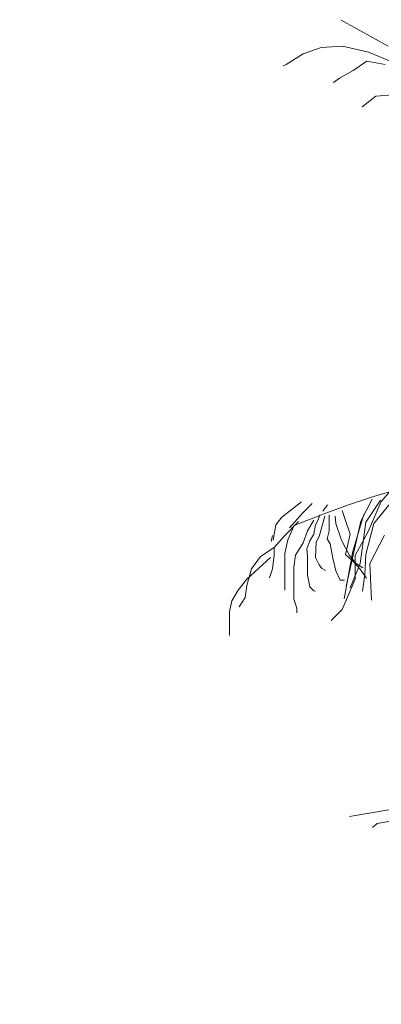
# Model space of a CAD drawing. Units: millimetres. Extents: x 595116 to 630915, y 909473 to 920225.
# Tile 33 of 134: x 629654.1 to 629660.18, y 919163.95 to 919180.52. Entities that reach past the tile are written whole.
import ezdxf

# ---------------------------------------------------------------- set-up
doc = ezdxf.new("R2010")
doc.units = ezdxf.units.MM
doc.layers.add('Dimension', color=3, linetype='Continuous', lineweight=18)
doc.layers.add('L-PLNT', color=85, linetype='Continuous', lineweight=13)
doc.styles.get("Standard").update_dxf_attribs({"font": 'arial.ttf'})
doc.dimstyles.new('ISO-25', dxfattribs={"dimtxt": 9, "dimasz": 6, "dimexe": 1.25, "dimexo": 0.625, "dimtad": 1, "dimlunit": 4, "dimtxsty": 'Standard', "dimcen": 2.5, "dimadec": 0, "dimazin": 0, "dimtfac": 1, "dimtmove": 0, "dimatfit": 3, "dimfxl": 1, "dimarcsym": 0})

# ---------------------------------------------------------------- blocks, each defined once
blk = doc.blocks.new('A$C4FB75ABC')
for p, q in [((0.4999, 4.2779), (0.7111, 4.1621)), ((0.4114, 4.1553), (0.3296, 4.1281)), ((0.5068, 4.1621), (0.4114, 4.1553)), ((0.6226, 4.1349), (0.5068, 4.1621)), ((0.3296, 4.1281), (0.2547, 4.0804)), ((0.7861, 4.0668), (0.6226, 4.1349)), ((0.2547, 4.0804), (0.241, 4.0736)), ((0.6158, 4.094), (0.5544, 4.0532)), ((0.6975, 4.0804), (0.6158, 4.094)), ((0.4931, 4.0191), (0.4659, 3.9987)), ((0.5544, 4.0532), (0.4931, 4.0191)), ((0.6566, 3.9374), (0.5953, 3.8897)), ((0.7316, 3.9442), (0.6566, 3.9374)), ((0.7572, 2.2091), (0.6795, 2.1218)), ((0.7422, 2.1723), (0.6405, 2.1416)), ((0.2683, 2.0784), (0.3228, 2.1193)), ((0.6405, 2.1416), (0.5342, 2.1057)), ((0.64, 2.1313), (0.5889, 2.0328)), ((0.6765, 2.1276), (0.6108, 2.0291)), ((0.6795, 2.1218), (0.6213, 1.986)), ((0.7531, 2.1531), (0.6473, 2.0218)), ((0.2342, 2.0512), (0.2683, 2.0784)), ((0.3296, 2.0716), (0.3705, 2.1125)), ((0.4182, 2.0784), (0.4386, 2.1057)), ((0.5342, 2.1057), (0.4195, 2.0639)), ((0.505, 2.0802), (0.5196, 2.0364)), ((0.207, 2.0172), (0.2342, 2.0512)), ((0.3092, 2.0308), (0.2479, 1.9695)), ((0.2683, 2.0035), (0.3296, 2.0716)), ((0.4195, 2.0639), (0.2927, 2.0154)), ((0.3773, 2.0376), (0.3501, 1.9899)), ((0.3966, 2.0361), (0.3855, 2.0168)), ((0.4049, 2.0609), (0.3966, 2.0361)), ((0.427, 2.0554), (0.4021, 1.9643)), ((0.4463, 2.0609), (0.4463, 1.9892)), ((0.4739, 2.0554), (0.4767, 2.0223)), ((0.5196, 2.0364), (0.5415, 1.9744)), ((0.5889, 2.0328), (0.5232, 1.741)), ((0.6018, 2.0636), (0.5533, 1.8986)), ((0.195, 1.9478), (0.207, 2.0172)), ((0.2887, 2.0103), (0.2615, 1.9491)), ((0.3501, 1.9899), (0.3296, 1.9354)), ((0.3855, 2.0168), (0.3773, 1.9754)), ((0.4463, 1.9892), (0.438, 1.9533)), ((0.4767, 2.0223), (0.5015, 1.9478)), ((0.6213, 1.986), (0.563, 1.8792)), ((0.6108, 2.0291), (0.5853, 1.8431)), ((0.6473, 2.0218), (0.6108, 1.8833)), ((0.1865, 1.9422), (0.1934, 1.9695)), ((0.2479, 1.9695), (0.2002, 1.915)), ((0.2615, 1.9491), (0.2479, 1.8878)), ((0.3607, 1.945), (0.3469, 1.9091)), ((0.3773, 1.9754), (0.3607, 1.945)), ((0.4021, 1.9643), (0.3883, 1.9395)), ((0.438, 1.9533), (0.4518, 1.9312)), ((0.5015, 1.9478), (0.5374, 1.8788)), ((0.5415, 1.9744), (0.5196, 1.8833)), ((0.6947, 1.9708), (0.629, 1.8431)), ((0.2002, 1.915), (0.1389, 1.8742)), ((0.2002, 1.915), (0.2002, 1.881)), ((0.3296, 1.9354), (0.2956, 1.881)), ((0.3469, 1.9091), (0.3497, 1.876)), ((0.3883, 1.9395), (0.3855, 1.8705)), ((0.4518, 1.9312), (0.4629, 1.8677)), ((0.5533, 1.8986), (0.5339, 1.7919)), ((0.1844, 1.8695), (0.0777, 1.7725)), ((0.1389, 1.8742), (0.098, 1.8197)), ((0.2002, 1.881), (0.1934, 1.8197)), ((0.2479, 1.8878), (0.2479, 1.8061)), ((0.2956, 1.881), (0.2887, 1.8265)), ((0.3497, 1.876), (0.3497, 1.8512)), ((0.3855, 1.8705), (0.4021, 1.8374)), ((0.4629, 1.8677), (0.4767, 1.8098)), ((0.5196, 1.8833), (0.5524, 1.8541)), ((0.5374, 1.8788), (0.5678, 1.8429)), ((0.5524, 1.8541), (0.5853, 1.8176)), ((0.563, 1.8792), (0.563, 1.7725)), ((0.6108, 1.8833), (0.6072, 1.7957)), ((0.098, 1.8197), (0.0775, 1.7448)), ((0.1934, 1.8197), (0.1797, 1.7788)), ((0.2887, 1.8265), (0.2887, 1.7516)), ((0.3497, 1.8512), (0.3497, 1.7904)), ((0.4021, 1.8374), (0.4132, 1.8208)), ((0.4132, 1.8208), (0.4297, 1.8125)), ((0.4767, 1.8098), (0.496, 1.7684)), ((0.5853, 1.8431), (0.5415, 1.7337)), ((0.5678, 1.8429), (0.5982, 1.8236)), ((0.5853, 1.8176), (0.6072, 1.7884)), ((0.629, 1.8431), (0.6363, 1.679)), ((0.0777, 1.7725), (0.0388, 1.724)), ((0.2479, 1.8061), (0.2479, 1.7448)), ((0.3497, 1.7904), (0.3607, 1.738)), ((0.496, 1.7684), (0.5153, 1.7684)), ((0.563, 1.7725), (0.5048, 1.6367)), ((0.5339, 1.7919), (0.5145, 1.6852)), ((0.6072, 1.7957), (0.5962, 1.7191)), ((0.6072, 1.7884), (0.6144, 1.7775)), ((0.0388, 1.724), (0.0097, 1.6755)), ((0.0775, 1.7448), (0.0707, 1.6903)), ((0.2479, 1.7448), (0.2479, 1.7243)), ((0.2887, 1.7516), (0.2887, 1.6835)), ((0.3607, 1.738), (0.3773, 1.7214)), ((0.3773, 1.7214), (0.3855, 1.7187)), ((0.0707, 1.6903), (0.0435, 1.6494)), ((0.2887, 1.6835), (0.3024, 1.6426)), ((0.0097, 1.6755), (0, 1.627)), ((0.3024, 1.6426), (0.3024, 1.6222)), ((0.5048, 1.6367), (0.4562, 1.5882)), ((0, 1.627), (0, 1.5494)), ((0, 1.5494), (0, 1.5203)), ((0.7236, 0.7411), (0.5379, 0.7092)), ((0.6621, 0.678), (0.6405, 0.6602)), ((0.7393, 0.6917), (0.6621, 0.678))]:
    blk.add_line(p, q)
blk = doc.blocks.new('*D216')
at = {"layer": 'Defpoints', "color": 0, "transparency": 16777216}
for p in [(629743.541, 919411.928), (629505.041, 919411.828), (629743.541, 918832.378)]:
    blk.add_point(p, dxfattribs=at)
at = {"layer": 'Dimension', "color": 0, "lineweight": -2, "transparency": 16777216}
for p, q in [((629505.041, 919411.203), (629505.041, 918831.128)), ((629743.541, 919411.303), (629743.541, 918831.128)), ((629511.041, 918832.378), (629737.541, 918832.378))]:
    blk.add_line(p, q, dxfattribs=at)
at = {"layer": 'Dimension', "color": 0, "transparency": 16777216}
for points in [[(629511.041, 918833.378), (629511.041, 918831.378), (629505.041, 918832.378)], [(629737.541, 918833.378), (629737.541, 918831.378), (629743.541, 918832.378)]]:
    blk.add_solid(points, dxfattribs=at)
at = {"layer": 'Dimension', "color": 0, "transparency": 16777216, "insert": (629624.291, 918837.656), "char_height": 9, "attachment_point": 5}
blk.add_mtext('19\'-10 1/2"', dxfattribs=at)

msp = doc.modelspace()

# ---------------------------------------------------------------- block references
at = {"layer": 'L-PLNT', "xscale": 3.753413438031968, "yscale": 3.753413438031968, "zscale": 3.753413438031968}
msp.add_blockref('A$C4FB75ABC', (629657.627, 919164.449), dxfattribs=at)

# ---------------------------------------------------------------- dimensions: what is measured, and where the dimension line sits
at = {"layer": 'Dimension'}
dim = msp.add_linear_dim(base=(629743.541, 918832.378), p1=(629505.041, 919411.828), p2=(629743.541, 919411.928), dimstyle='ISO-25', override={"dimdec": 1, "dimlfac": 1, "dimrnd": 0, "dimzin": 1, "dimdsep": 46, "dimlunit": 4, "dimfrac": 2}, dxfattribs=at)
dim.commit()
dim.dimension.update_dxf_attribs({"geometry": '*D216', "text_midpoint": (629624.291, 918837.656)})

doc.saveas('drawing.dxf')
